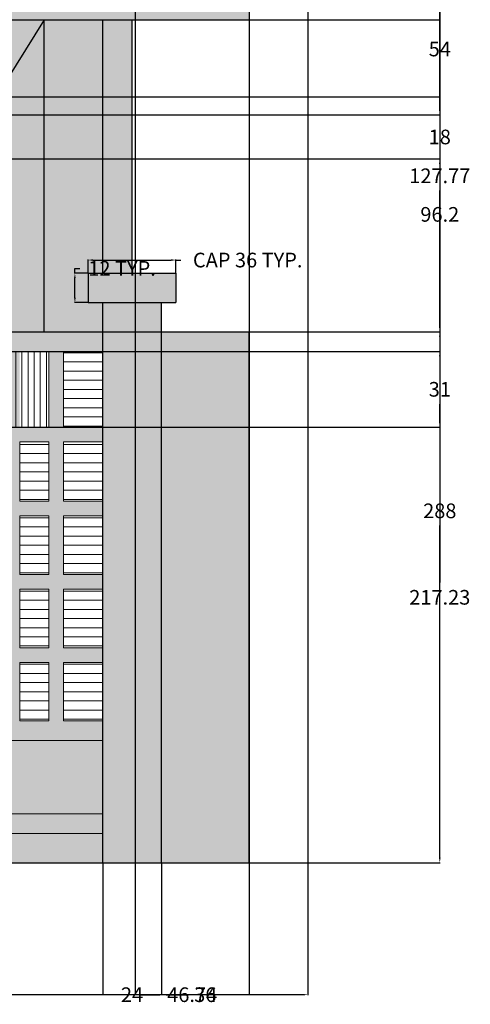
# Model space of a CAD drawing. Units: inches. Extents: x 180 to 1069, y 71 to 1267.
# Tile 5 of 8: x 884 to 1069, y 71 to 474. Entities that reach past the tile are written whole.
import ezdxf

# ---------------------------------------------------------------- set-up
doc = ezdxf.new("R2010")
doc.units = ezdxf.units.IN
doc.header["$MEASUREMENT"] = 0
for name, color, linetype, lineweight in [('A-ANNO-DIMS', 2, 'Continuous', 18), ('A-COLS', 7, 'Continuous', 25), ('A-DOOR-GATE', 7, 'Continuous', 18), ('A-DOOR-PANL-PATT', 25, 'Continuous', 13), ('A-WALL', 7, 'Continuous', 30)]:
    doc.layers.add(name, color=color, linetype=linetype, lineweight=lineweight)
for name, color, linetype, lineweight, true_color in [('A-DOOR-GATE-PATT', 18, 'Continuous', 13, 0x000000), ('A-DOOR-HARD-PATT', 8, 'Continuous', 13, 0x7f7f6c), ('A-ELEV-FRAM-PATT', 53, 'Continuous', 13, 0xefd648), ('A-ELEV-REVL-PATT', 9, 'Continuous', 13, 0xc7c8ca), ('A-ELEV-TRIM-PATT', 7, 'Continuous', 13, 0xffffff), ('A-WALL-PATT', 253, 'Continuous', 13, 0x9f9f8e), ('A-WALL-RCSD-PATT', 251, 'Continuous', 13, 0x696959)]:
    doc.layers.add(name, color=color, linetype=linetype, lineweight=lineweight, true_color=true_color)
doc.styles.get("Standard").update_dxf_attribs({"font": 'arial.ttf'})
doc.dimstyles.get("Standard").update_dxf_attribs({"dimtxt": 6, "dimasz": 2, "dimexe": 0.18, "dimexo": 0.0625, "dimgap": 3, "dimtad": 0, "dimtih": 1, "dimtoh": 1, "dimdec": 0, "dimzin": 0, "dimdsep": 46, "dimlunit": 3, "dimtxsty": 'Standard', "dimcen": 0.09, "dimadec": 0, "dimazin": 0, "dimtfac": 1, "dimtdec": 0, "dimtofl": 0, "dimtmove": 0, "dimatfit": 3, "dimfxl": 1, "dimtolj": 1, "dimtzin": 0, "dimarcsym": 0})

# ---------------------------------------------------------------- blocks, each defined once
blk = doc.blocks.new('GATE-PIER-CAP')
for p, q in [((0, 12), (36, 12)), ((0, 12), (0, 0)), ((36, 12), (36, 0)), ((0, 0), (36, 0))]:
    blk.add_line(p, q)
blk = doc.blocks.new('GATE-LEAF-LOWER-INFILL')
for p, q in [((0, 152.23), (16, 152.23)), ((16, 152.23), (16, 128)), ((22, 152.23), (34, 152.23)), ((22, 152.23), (22, 128)), ((34, 152.23), (34, 128)), ((40, 152.23), (88, 152.23)), ((40, 152.23), (40, 128)), ((88, 152.23), (88, 128)), ((94, 152.23), (106, 152.23)), ((94, 152.23), (94, 128)), ((106, 152.23), (106, 128)), ((112, 152.23), (136, 152.23)), ((112, 152.23), (112, 128)), ((136, 152.23), (136, 128)), ((0, 128), (16, 128)), ((22, 128), (34, 128)), ((40, 128), (88, 128)), ((94, 128), (106, 128)), ((112, 128), (136, 128)), ((0, 122), (16, 122)), ((16, 122), (16, 98)), ((22, 122), (34, 122)), ((22, 122), (22, 98)), ((34, 122), (34, 98)), ((40, 122), (88, 122)), ((40, 122), (40, 98)), ((88, 122), (88, 98)), ((94, 122), (106, 122)), ((94, 122), (94, 98)), ((106, 122), (106, 98)), ((112, 122), (136, 122)), ((112, 122), (112, 98)), ((136, 122), (136, 98)), ((0, 98), (16, 98)), ((22, 98), (34, 98)), ((40, 98), (88, 98)), ((94, 98), (106, 98)), ((112, 98), (136, 98)), ((0, 92), (16, 92)), ((16, 92), (16, 68)), ((22, 92), (34, 92)), ((22, 92), (22, 68)), ((34, 92), (34, 68)), ((40, 92), (88, 92)), ((40, 92), (40, 68)), ((88, 92), (88, 68)), ((94, 92), (106, 92)), ((94, 92), (94, 68)), ((106, 92), (106, 68)), ((112, 92), (136, 92)), ((112, 92), (112, 68)), ((136, 92), (136, 68)), ((0, 68), (16, 68)), ((22, 68), (34, 68)), ((40, 68), (88, 68)), ((94, 68), (106, 68)), ((112, 68), (136, 68)), ((0, 62), (16, 62)), ((16, 62), (16, 38)), ((22, 62), (34, 62)), ((22, 62), (22, 38)), ((34, 62), (34, 38)), ((40, 62), (88, 62)), ((40, 62), (40, 38)), ((88, 62), (88, 38)), ((94, 62), (106, 62)), ((94, 62), (94, 38)), ((106, 62), (106, 38)), ((112, 62), (136, 62)), ((112, 62), (112, 38)), ((136, 62), (136, 38)), ((0, 38), (16, 38)), ((22, 38), (34, 38)), ((40, 38), (88, 38)), ((94, 38), (106, 38)), ((112, 38), (136, 38)), ((0, 30), (136, 30)), ((136, 30), (136, 0)), ((0, 0), (136, 0))]:
    blk.add_line(p, q)
blk = doc.blocks.new('*D12')
at = {"layer": 'A-ANNO-DIMS', "color": 0, "lineweight": -2, "transparency": 16777216}
for p, q in [((912.09, 370.11), (912.09, 375.63)), ((914.09, 375.45), (946.09, 375.45)), ((948.09, 370.11), (948.09, 375.63)), ((948.09, 375.45), (950.09, 375.45))]:
    blk.add_line(p, q, dxfattribs=at)
at = {"layer": 'A-ANNO-DIMS', "color": 0, "transparency": 16777216}
for points in [[(914.09, 375.78), (914.09, 375.11), (912.09, 375.45)], [(946.09, 375.78), (946.09, 375.11), (948.09, 375.45)]]:
    blk.add_solid(points, dxfattribs=at)
at = {"layer": 'Defpoints', "color": 0, "transparency": 16777216}
for p in [(948.09, 375.45), (912.09, 370.05), (948.09, 370.05)]:
    blk.add_point(p, dxfattribs=at)
at = {"layer": 'A-ANNO-DIMS', "color": 0, "transparency": 16777216, "insert": (977.44, 375.45), "char_height": 6, "attachment_point": 5}
blk.add_mtext('\\A1;CAP 36 TYP.', dxfattribs=at)
blk = doc.blocks.new('*D13')
at = {"layer": 'A-ANNO-DIMS', "color": 0, "lineweight": -2, "transparency": 16777216}
for p, q in [((906.69, 370.05), (906.69, 372.05)), ((906.69, 372.05), (908.69, 372.05)), ((912.02, 370.05), (906.51, 370.05)), ((906.69, 360.05), (906.69, 368.05)), ((912.02, 358.05), (906.51, 358.05))]:
    blk.add_line(p, q, dxfattribs=at)
at = {"layer": 'A-ANNO-DIMS', "color": 0, "transparency": 16777216}
for points in [[(906.35, 368.05), (907.02, 368.05), (906.69, 370.05)], [(906.35, 360.05), (907.02, 360.05), (906.69, 358.05)]]:
    blk.add_solid(points, dxfattribs=at)
at = {"layer": 'Defpoints', "color": 0, "transparency": 16777216}
for p in [(906.69, 370.05), (912.09, 370.05), (912.09, 358.05)]:
    blk.add_point(p, dxfattribs=at)
at = {"layer": 'A-ANNO-DIMS', "color": 0, "transparency": 16777216, "insert": (926.01, 372.05), "char_height": 6, "attachment_point": 5}
blk.add_mtext('\\A1;12 TYP.', dxfattribs=at)
blk = doc.blocks.new('*D31')
at = {"layer": 'A-ANNO-DIMS', "color": 0, "lineweight": -2, "transparency": 16777216}
for p, q in [((546.15, 416.82), (1056.28, 416.82)), ((1056.1, 414.82), (1056.1, 278.88)), ((1056.1, 130.82), (1056.1, 266.75)), ((546.15, 128.82), (1056.28, 128.82))]:
    blk.add_line(p, q, dxfattribs=at)
at = {"layer": 'A-ANNO-DIMS', "color": 0, "transparency": 16777216}
for points in [[(1055.77, 414.82), (1056.43, 414.82), (1056.1, 416.82)], [(1055.77, 130.82), (1056.43, 130.82), (1056.1, 128.82)]]:
    blk.add_solid(points, dxfattribs=at)
at = {"layer": 'Defpoints', "color": 0, "transparency": 16777216}
for p in [(546.09, 416.82), (1056.1, 416.82), (546.09, 128.82)]:
    blk.add_point(p, dxfattribs=at)
at = {"layer": 'A-ANNO-DIMS', "color": 0, "transparency": 16777216, "insert": (1056.1, 272.82), "char_height": 6, "attachment_point": 5}
blk.add_mtext('\\A1;288', dxfattribs=at)
blk = doc.blocks.new('*D32')
at = {"layer": 'A-ANNO-DIMS', "color": 0, "lineweight": -2, "transparency": 16777216}
for p, q in [((1056.1, 436.82), (1056.1, 438.82)), ((606.15, 434.82), (1056.28, 434.82)), ((546.15, 416.82), (1056.28, 416.82)), ((1056.1, 414.82), (1056.1, 412.82))]:
    blk.add_line(p, q, dxfattribs=at)
at = {"layer": 'A-ANNO-DIMS', "color": 0, "transparency": 16777216}
for points in [[(1055.77, 436.82), (1056.43, 436.82), (1056.1, 434.82)], [(1055.77, 414.82), (1056.43, 414.82), (1056.1, 416.82)]]:
    blk.add_solid(points, dxfattribs=at)
at = {"layer": 'Defpoints', "color": 0, "transparency": 16777216}
for p in [(606.09, 434.82), (1056.1, 434.82), (546.09, 416.82)]:
    blk.add_point(p, dxfattribs=at)
at = {"layer": 'A-ANNO-DIMS', "color": 0, "transparency": 16777216, "insert": (1056.1, 425.82), "char_height": 6, "attachment_point": 5}
blk.add_mtext('\\A1;18', dxfattribs=at)
blk = doc.blocks.new('*D34')
at = {"layer": 'A-ANNO-DIMS', "color": 0, "lineweight": -2, "transparency": 16777216}
for p, q in [((630.09, 128.75), (630.09, 74.62)), ((918.09, 128.75), (918.09, 74.62)), ((632.09, 74.8), (764.4, 74.8)), ((916.09, 74.8), (783.77, 74.8))]:
    blk.add_line(p, q, dxfattribs=at)
at = {"layer": 'A-ANNO-DIMS', "color": 0, "transparency": 16777216}
for points in [[(632.09, 75.14), (632.09, 74.47), (630.09, 74.8)], [(916.09, 75.14), (916.09, 74.47), (918.09, 74.8)]]:
    blk.add_solid(points, dxfattribs=at)
at = {"layer": 'Defpoints', "color": 0, "transparency": 16777216}
for p in [(630.09, 128.82), (918.09, 128.82), (918.09, 74.8)]:
    blk.add_point(p, dxfattribs=at)
at = {"layer": 'A-ANNO-DIMS', "color": 0, "transparency": 16777216, "insert": (774.09, 74.8), "char_height": 6, "attachment_point": 5}
blk.add_mtext('\\A1;288', dxfattribs=at)
blk = doc.blocks.new('*D35')
at = {"layer": 'A-ANNO-DIMS', "color": 0, "lineweight": -2, "transparency": 16777216}
for p, q in [((918.09, 128.75), (918.09, 74.62)), ((942.09, 128.75), (942.09, 74.62)), ((916.09, 74.8), (914.09, 74.8)), ((944.09, 74.8), (946.09, 74.8))]:
    blk.add_line(p, q, dxfattribs=at)
at = {"layer": 'A-ANNO-DIMS', "color": 0, "transparency": 16777216}
for points in [[(916.09, 75.14), (916.09, 74.47), (918.09, 74.8)], [(944.09, 75.14), (944.09, 74.47), (942.09, 74.8)]]:
    blk.add_solid(points, dxfattribs=at)
at = {"layer": 'Defpoints', "color": 0, "transparency": 16777216}
for p in [(918.09, 128.82), (942.09, 128.82), (942.09, 74.8)]:
    blk.add_point(p, dxfattribs=at)
at = {"layer": 'A-ANNO-DIMS', "color": 0, "transparency": 16777216, "insert": (930.09, 74.8), "char_height": 6, "attachment_point": 5}
blk.add_mtext('\\A1;24', dxfattribs=at)
blk = doc.blocks.new('*D36')
at = {"layer": 'A-ANNO-DIMS', "color": 0, "lineweight": -2, "transparency": 16777216}
for p, q in [((942.09, 128.75), (942.09, 74.62)), ((978.09, 128.75), (978.09, 74.62)), ((944.09, 74.8), (952.79, 74.8)), ((976.09, 74.8), (967.38, 74.8))]:
    blk.add_line(p, q, dxfattribs=at)
at = {"layer": 'A-ANNO-DIMS', "color": 0, "transparency": 16777216}
for points in [[(944.09, 75.14), (944.09, 74.47), (942.09, 74.8)], [(976.09, 75.14), (976.09, 74.47), (978.09, 74.8)]]:
    blk.add_solid(points, dxfattribs=at)
at = {"layer": 'Defpoints', "color": 0, "transparency": 16777216}
for p in [(942.09, 128.82), (978.09, 128.82), (978.09, 74.8)]:
    blk.add_point(p, dxfattribs=at)
at = {"layer": 'A-ANNO-DIMS', "color": 0, "transparency": 16777216, "insert": (960.09, 74.8), "char_height": 6, "attachment_point": 5}
blk.add_mtext('\\A1;36', dxfattribs=at)
blk = doc.blocks.new('*D37')
at = {"layer": 'A-ANNO-DIMS', "color": 0, "lineweight": -2, "transparency": 16777216}
for p, q in [((978.15, 346.05), (1056.28, 346.05)), ((1056.1, 344.05), (1056.1, 243.5)), ((1056.1, 130.82), (1056.1, 231.37)), ((978.15, 128.82), (1056.28, 128.82))]:
    blk.add_line(p, q, dxfattribs=at)
at = {"layer": 'A-ANNO-DIMS', "color": 0, "transparency": 16777216}
for points in [[(1055.77, 344.05), (1056.43, 344.05), (1056.1, 346.05)], [(1055.77, 130.82), (1056.43, 130.82), (1056.1, 128.82)]]:
    blk.add_solid(points, dxfattribs=at)
at = {"layer": 'Defpoints', "color": 0, "transparency": 16777216}
for p in [(978.09, 346.05), (1056.1, 346.05), (978.09, 128.82)]:
    blk.add_point(p, dxfattribs=at)
at = {"layer": 'A-ANNO-DIMS', "color": 0, "transparency": 16777216, "insert": (1056.1, 237.43), "char_height": 6, "attachment_point": 5}
blk.add_mtext('\\A1;217.23', dxfattribs=at)
blk = doc.blocks.new('*D38')
at = {"layer": 'A-ANNO-DIMS', "color": 0, "lineweight": -2, "transparency": 16777216}
for p, q in [((978.15, 473.82), (1056.28, 473.82)), ((1056.1, 471.82), (1056.1, 415.94)), ((1056.1, 348.05), (1056.1, 403.92)), ((978.15, 346.05), (1056.28, 346.05))]:
    blk.add_line(p, q, dxfattribs=at)
at = {"layer": 'A-ANNO-DIMS', "color": 0, "transparency": 16777216}
for points in [[(1055.77, 471.82), (1056.43, 471.82), (1056.1, 473.82)], [(1055.77, 348.05), (1056.43, 348.05), (1056.1, 346.05)]]:
    blk.add_solid(points, dxfattribs=at)
at = {"layer": 'Defpoints', "color": 0, "transparency": 16777216}
for p in [(978.09, 473.82), (1056.1, 473.82), (978.09, 346.05)]:
    blk.add_point(p, dxfattribs=at)
at = {"layer": 'A-ANNO-DIMS', "color": 0, "transparency": 16777216, "insert": (1056.1, 409.93), "char_height": 6, "attachment_point": 5}
blk.add_mtext('\\A1;127.77', dxfattribs=at)
blk = doc.blocks.new('*D41')
at = {"layer": 'A-ANNO-DIMS', "color": 0, "lineweight": -2, "transparency": 16777216}
for p, q in [((736.15, 338.05), (1056.28, 338.05)), ((1056.1, 336.05), (1056.1, 328.61)), ((1056.1, 309.05), (1056.1, 316.48)), ((736.15, 307.05), (1056.28, 307.05))]:
    blk.add_line(p, q, dxfattribs=at)
at = {"layer": 'A-ANNO-DIMS', "color": 0, "transparency": 16777216}
for points in [[(1055.77, 336.05), (1056.43, 336.05), (1056.1, 338.05)], [(1055.77, 309.05), (1056.43, 309.05), (1056.1, 307.05)]]:
    blk.add_solid(points, dxfattribs=at)
at = {"layer": 'Defpoints', "color": 0, "transparency": 16777216}
for p in [(736.09, 338.05), (736.09, 307.05), (1056.1, 307.05)]:
    blk.add_point(p, dxfattribs=at)
at = {"layer": 'A-ANNO-DIMS', "color": 0, "transparency": 16777216, "insert": (1056.1, 322.55), "char_height": 6, "attachment_point": 5}
blk.add_mtext('\\A1;31', dxfattribs=at)
blk = doc.blocks.new('*D47')
at = {"layer": 'A-ANNO-DIMS', "color": 0, "lineweight": -2, "transparency": 16777216}
for p, q in [((825.96, 442.24), (1056.28, 442.24)), ((1056.1, 440.24), (1056.1, 400.21)), ((1056.1, 348.05), (1056.1, 388.08)), ((825.96, 346.05), (1056.28, 346.05))]:
    blk.add_line(p, q, dxfattribs=at)
at = {"layer": 'A-ANNO-DIMS', "color": 0, "transparency": 16777216}
for points in [[(1055.77, 440.24), (1056.43, 440.24), (1056.1, 442.24)], [(1055.77, 348.05), (1056.43, 348.05), (1056.1, 346.05)]]:
    blk.add_solid(points, dxfattribs=at)
at = {"layer": 'Defpoints', "color": 0, "transparency": 16777216}
for p in [(825.89, 442.24), (1056.1, 442.24), (825.89, 346.05)]:
    blk.add_point(p, dxfattribs=at)
at = {"layer": 'A-ANNO-DIMS', "color": 0, "transparency": 16777216, "insert": (1056.1, 394.14), "char_height": 6, "attachment_point": 5}
blk.add_mtext('\\A1;96.2', dxfattribs=at)
blk = doc.blocks.new('*D59')
at = {"layer": 'A-ANNO-DIMS', "color": 0, "lineweight": -2, "transparency": 16777216}
for p, q in [((606.15, 1010.82), (1056.28, 1010.82)), ((1056.1, 1008.82), (1056.1, 728.88)), ((1056.1, 436.82), (1056.1, 716.75)), ((606.15, 434.82), (1056.28, 434.82))]:
    blk.add_line(p, q, dxfattribs=at)
at = {"layer": 'A-ANNO-DIMS', "color": 0, "transparency": 16777216}
for points in [[(1055.77, 1008.82), (1056.43, 1008.82), (1056.1, 1010.82)], [(1055.77, 436.82), (1056.43, 436.82), (1056.1, 434.82)]]:
    blk.add_solid(points, dxfattribs=at)
at = {"layer": 'Defpoints', "color": 0, "transparency": 16777216}
for p in [(606.09, 1010.82), (1056.1, 1010.82), (606.09, 434.82)]:
    blk.add_point(p, dxfattribs=at)
at = {"layer": 'A-ANNO-DIMS', "color": 0, "transparency": 16777216, "insert": (1056.1, 722.82), "char_height": 6, "attachment_point": 5}
blk.add_mtext('\\A1;576', dxfattribs=at)
blk = doc.blocks.new('*D60')
at = {"layer": 'A-ANNO-DIMS', "color": 0, "lineweight": -2, "transparency": 16777216}
for p, q in [((498.15, 488.82), (1056.28, 488.82)), ((1056.1, 486.82), (1056.1, 467.87)), ((1056.1, 436.82), (1056.1, 455.76)), ((606.15, 434.82), (1056.28, 434.82))]:
    blk.add_line(p, q, dxfattribs=at)
at = {"layer": 'A-ANNO-DIMS', "color": 0, "transparency": 16777216}
for points in [[(1055.77, 486.82), (1056.43, 486.82), (1056.1, 488.82)], [(1055.77, 436.82), (1056.43, 436.82), (1056.1, 434.82)]]:
    blk.add_solid(points, dxfattribs=at)
at = {"layer": 'Defpoints', "color": 0, "transparency": 16777216}
for p in [(498.09, 488.82), (606.09, 434.82), (1056.1, 434.82)]:
    blk.add_point(p, dxfattribs=at)
at = {"layer": 'A-ANNO-DIMS', "color": 0, "transparency": 16777216, "insert": (1056.1, 461.82), "char_height": 6, "attachment_point": 5}
blk.add_mtext('\\A1;54', dxfattribs=at)
blk = doc.blocks.new('*D68')
at = {"layer": 'A-ANNO-DIMS', "color": 0, "lineweight": -2, "transparency": 16777216}
for p, q in [((702.09, 557.75), (702.09, 74.62)), ((1002.09, 557.75), (1002.09, 74.62)), ((704.09, 74.8), (842.47, 74.8)), ((1000.09, 74.8), (861.7, 74.8))]:
    blk.add_line(p, q, dxfattribs=at)
at = {"layer": 'A-ANNO-DIMS', "color": 0, "transparency": 16777216}
for points in [[(704.09, 75.14), (704.09, 74.47), (702.09, 74.8)], [(1000.09, 75.14), (1000.09, 74.47), (1002.09, 74.8)]]:
    blk.add_solid(points, dxfattribs=at)
at = {"layer": 'Defpoints', "color": 0, "transparency": 16777216}
for p in [(702.09, 557.82), (1002.09, 557.82), (1002.09, 74.8)]:
    blk.add_point(p, dxfattribs=at)
at = {"layer": 'A-ANNO-DIMS', "color": 0, "transparency": 16777216, "insert": (852.09, 74.8), "char_height": 6, "attachment_point": 5}
blk.add_mtext('\\A1;300', dxfattribs=at)
blk = doc.blocks.new('*D79')
at = {"layer": 'A-ANNO-DIMS', "color": 0, "lineweight": -2, "transparency": 16777216}
for p, q in [((931.35, 647.75), (931.35, 74.62)), ((978.09, 647.75), (978.09, 74.62)), ((933.35, 74.8), (941.49, 74.8)), ((976.09, 74.8), (967.95, 74.8))]:
    blk.add_line(p, q, dxfattribs=at)
at = {"layer": 'A-ANNO-DIMS', "color": 0, "transparency": 16777216}
for points in [[(933.35, 75.14), (933.35, 74.47), (931.35, 74.8)], [(976.09, 75.14), (976.09, 74.47), (978.09, 74.8)]]:
    blk.add_solid(points, dxfattribs=at)
at = {"layer": 'Defpoints', "color": 0, "transparency": 16777216}
for p in [(931.35, 647.82), (978.09, 647.82), (978.09, 74.8)]:
    blk.add_point(p, dxfattribs=at)
at = {"layer": 'A-ANNO-DIMS', "color": 0, "transparency": 16777216, "insert": (954.72, 74.8), "char_height": 6, "attachment_point": 5}
blk.add_mtext('\\A1;46.74', dxfattribs=at)

msp = doc.modelspace()

# ---------------------------------------------------------------- hatches: boundary and pattern name
at = {"layer": 'A-DOOR-GATE-PATT'}
h = msp.add_hatch(color=256, dxfattribs=at)
h.dxf.hatch_style = 1
h.paths.add_polyline_path([(772.0875, 346.0477), (630.0875, 346.0477), (630.0875, 338.0477), (646.0875, 338.0477), (646.0875, 307.0477), (630.0875, 307.0477), (630.0875, 301.0477), (646.0875, 301.0477), (646.0875, 276.8159), (630.0875, 276.8159), (630.0875, 270.8159), (646.0875, 270.8159), (646.0875, 246.8159), (630.0875, 246.8159), (630.0875, 240.8159), (646.0875, 240.8159), (646.0875, 216.8159), (630.0875, 216.8159), (630.0875, 210.8159), (646.0875, 210.8159), (646.0875, 186.8159), (630.0875, 186.8159), (630.0875, 178.8159), (766.0875, 178.8159), (766.0875, 148.8159), (630.0875, 148.8159), (630.0875, 140.8159), (772.0875, 140.8159)])
h.paths.add_polyline_path([(670.0875, 338.0477), (718.0875, 338.0477), (718.0875, 307.0477), (670.0875, 307.0477)], flags=16)
h.paths.add_polyline_path([(664.0875, 338.0477), (664.0875, 307.0477), (652.0875, 307.0477), (652.0875, 338.0477)], flags=16)
h.paths.add_polyline_path([(670.0875, 301.0477), (718.0875, 301.0477), (718.0875, 276.8159), (670.0875, 276.8159)], flags=16)
h.paths.add_polyline_path([(664.0875, 301.0477), (664.0875, 276.8159), (652.0875, 276.8159), (652.0875, 301.0477)], flags=16)
h.paths.add_polyline_path([(724.0875, 338.0477), (736.0875, 338.0477), (736.0875, 307.0477), (724.0875, 307.0477)], flags=16)
h.paths.add_polyline_path([(724.0875, 301.0477), (736.0875, 301.0477), (736.0875, 276.8159), (724.0875, 276.8159)], flags=16)
h.paths.add_polyline_path([(670.0875, 270.8159), (718.0875, 270.8159), (718.0875, 246.8159), (670.0875, 246.8159)], flags=16)
h.paths.add_polyline_path([(664.0875, 270.8159), (664.0875, 246.8159), (652.0875, 246.8159), (652.0875, 270.8159)], flags=16)
h.paths.add_polyline_path([(742.0875, 338.0477), (766.0875, 338.0477), (766.0875, 307.0477), (742.0875, 307.0477)], flags=16)
h.paths.add_polyline_path([(742.0875, 301.0477), (766.0875, 301.0477), (766.0875, 276.8159), (742.0875, 276.8159)], flags=16)
h.paths.add_polyline_path([(724.0875, 270.8159), (736.0875, 270.8159), (736.0875, 246.8159), (724.0875, 246.8159)], flags=16)
h.paths.add_polyline_path([(670.0875, 240.8159), (718.0875, 240.8159), (718.0875, 216.8159), (670.0875, 216.8159)], flags=16)
h.paths.add_polyline_path([(664.0875, 240.8159), (664.0875, 216.8159), (652.0875, 216.8159), (652.0875, 240.8159)], flags=16)
h.paths.add_polyline_path([(742.0875, 270.8159), (766.0875, 270.8159), (766.0875, 246.8159), (742.0875, 246.8159)], flags=16)
h.paths.add_polyline_path([(724.0875, 240.8159), (736.0875, 240.8159), (736.0875, 216.8159), (724.0875, 216.8159)], flags=16)
h.paths.add_polyline_path([(742.0875, 240.8159), (766.0875, 240.8159), (766.0875, 216.8159), (742.0875, 216.8159)], flags=16)
h.paths.add_polyline_path([(670.0875, 210.8159), (718.0875, 210.8159), (718.0875, 186.8159), (670.0875, 186.8159)], flags=16)
h.paths.add_polyline_path([(664.0875, 210.8159), (664.0875, 186.8159), (652.0875, 186.8159), (652.0875, 210.8159)], flags=16)
h.paths.add_polyline_path([(724.0875, 210.8159), (736.0875, 210.8159), (736.0875, 186.8159), (724.0875, 186.8159)], flags=16)
h.paths.add_polyline_path([(742.0875, 210.8159), (766.0875, 210.8159), (766.0875, 186.8159), (742.0875, 186.8159)], flags=16)
h.paths.add_polyline_path([(918.0875, 346.0477), (776.0875, 346.0477), (776.0875, 140.8159), (918.0875, 140.8159), (918.0875, 148.8159), (782.0875, 148.8159), (782.0875, 178.8159), (918.0875, 178.8159), (918.0875, 186.8159), (902.0875, 186.8159), (902.0875, 210.8159), (918.0875, 210.8159), (918.0875, 216.8159), (902.0875, 216.8159), (902.0875, 240.8159), (918.0875, 240.8159), (918.0875, 246.8159), (902.0875, 246.8159), (902.0875, 270.8159), (918.0875, 270.8159), (918.0875, 276.8159), (902.0875, 276.8159), (902.0875, 301.0477), (918.0875, 301.0477), (918.0875, 307.0477), (902.0875, 307.0477), (902.0875, 338.0477), (918.0875, 338.0477)])
h.paths.add_polyline_path([(782.0875, 338.0477), (806.0875, 338.0477), (806.0875, 307.0477), (782.0875, 307.0477)], flags=16)
h.paths.add_polyline_path([(812.0875, 338.0477), (824.0875, 338.0477), (824.0875, 307.0477), (812.0875, 307.0477)], flags=16)
h.paths.add_polyline_path([(782.0875, 301.0477), (806.0875, 301.0477), (806.0875, 276.8159), (782.0875, 276.8159)], flags=16)
h.paths.add_polyline_path([(830.0875, 338.0477), (878.0875, 338.0477), (878.0875, 307.0477), (830.0875, 307.0477)], flags=16)
h.paths.add_polyline_path([(812.0875, 301.0477), (824.0875, 301.0477), (824.0875, 276.8159), (812.0875, 276.8159)], flags=16)
h.paths.add_polyline_path([(830.0875, 301.0477), (878.0875, 301.0477), (878.0875, 276.8159), (830.0875, 276.8159)], flags=16)
h.paths.add_polyline_path([(782.0875, 270.8159), (806.0875, 270.8159), (806.0875, 246.8159), (782.0875, 246.8159)], flags=16)
h.paths.add_polyline_path([(812.0875, 270.8159), (824.0875, 270.8159), (824.0875, 246.8159), (812.0875, 246.8159)], flags=16)
h.paths.add_polyline_path([(830.0875, 270.8159), (878.0875, 270.8159), (878.0875, 246.8159), (830.0875, 246.8159)], flags=16)
h.paths.add_polyline_path([(782.0875, 240.8159), (806.0875, 240.8159), (806.0875, 216.8159), (782.0875, 216.8159)], flags=16)
h.paths.add_polyline_path([(884.0875, 338.0477), (896.0875, 338.0477), (896.0875, 307.0477), (884.0875, 307.0477)], flags=16)
h.paths.add_polyline_path([(812.0875, 240.8159), (824.0875, 240.8159), (824.0875, 216.8159), (812.0875, 216.8159)], flags=16)
h.paths.add_polyline_path([(884.0875, 301.0477), (896.0875, 301.0477), (896.0875, 276.8159), (884.0875, 276.8159)], flags=16)
h.paths.add_polyline_path([(830.0875, 240.8159), (878.0875, 240.8159), (878.0875, 216.8159), (830.0875, 216.8159)], flags=16)
h.paths.add_polyline_path([(884.0875, 270.8159), (896.0875, 270.8159), (896.0875, 246.8159), (884.0875, 246.8159)], flags=16)
h.paths.add_polyline_path([(782.0875, 210.8159), (806.0875, 210.8159), (806.0875, 186.8159), (782.0875, 186.8159)], flags=16)
h.paths.add_polyline_path([(812.0875, 210.8159), (824.0875, 210.8159), (824.0875, 186.8159), (812.0875, 186.8159)], flags=16)
h.paths.add_polyline_path([(830.0875, 210.8159), (878.0875, 210.8159), (878.0875, 186.8159), (830.0875, 186.8159)], flags=16)
h.paths.add_polyline_path([(884.0875, 240.8159), (896.0875, 240.8159), (896.0875, 216.8159), (884.0875, 216.8159)], flags=16)
h.paths.add_polyline_path([(884.0875, 210.8159), (896.0875, 210.8159), (896.0875, 186.8159), (884.0875, 186.8159)], flags=16)
h = msp.add_hatch(dxfattribs=at)
h.set_pattern_fill('ANSI31', color=256, scale=30, angle=135)
h.paths.add_polyline_path([(646.0875, 338.0477), (630.0875, 338.0477), (630.0875, 307.0477), (646.0875, 307.0477)])
h.paths.add_polyline_path([(646.0875, 301.0477), (630.0875, 301.0477), (630.0875, 276.8159), (646.0875, 276.8159)])
h.paths.add_polyline_path([(664.0875, 301.0477), (652.0875, 301.0477), (652.0875, 276.8159), (664.0875, 276.8159)])
h.paths.add_polyline_path([(664.0875, 270.8159), (652.0875, 270.8159), (652.0875, 246.8159), (664.0875, 246.8159)])
h.paths.add_polyline_path([(646.0875, 270.8159), (630.0875, 270.8159), (630.0875, 246.8159), (646.0875, 246.8159)])
h.paths.add_polyline_path([(646.0875, 240.8159), (630.0875, 240.8159), (630.0875, 216.8159), (646.0875, 216.8159)])
h.paths.add_polyline_path([(664.0875, 240.8159), (652.0875, 240.8159), (652.0875, 216.8159), (664.0875, 216.8159)])
h.paths.add_polyline_path([(664.0875, 210.8159), (652.0875, 210.8159), (652.0875, 186.8159), (664.0875, 186.8159)])
h.paths.add_polyline_path([(646.0875, 210.8159), (630.0875, 210.8159), (630.0875, 186.8159), (646.0875, 186.8159)])
h.paths.add_polyline_path([(736.0875, 301.0477), (724.0875, 301.0477), (724.0875, 276.8159), (736.0875, 276.8159)])
h.paths.add_polyline_path([(766.0875, 301.0477), (742.0875, 301.0477), (742.0875, 276.8159), (766.0875, 276.8159)])
h.paths.add_polyline_path([(766.0875, 270.8159), (742.0875, 270.8159), (742.0875, 246.8159), (766.0875, 246.8159)])
h.paths.add_polyline_path([(766.0875, 338.0477), (742.0875, 338.0477), (742.0875, 307.0477), (766.0875, 307.0477)])
h.paths.add_polyline_path([(736.0875, 270.8159), (724.0875, 270.8159), (724.0875, 246.8159), (736.0875, 246.8159)])
h.paths.add_polyline_path([(736.0875, 240.8159), (724.0875, 240.8159), (724.0875, 216.8159), (736.0875, 216.8159)])
h.paths.add_polyline_path([(766.0875, 240.8159), (742.0875, 240.8159), (742.0875, 216.8159), (766.0875, 216.8159)])
h.paths.add_polyline_path([(766.0875, 210.8159), (742.0875, 210.8159), (742.0875, 186.8159), (766.0875, 186.8159)])
h.paths.add_polyline_path([(736.0875, 210.8159), (724.0875, 210.8159), (724.0875, 186.8159), (736.0875, 186.8159)])
h.paths.add_polyline_path([(806.0875, 210.8159), (782.0875, 210.8159), (782.0875, 186.8159), (806.0875, 186.8159)])
h.paths.add_polyline_path([(806.0875, 240.8159), (782.0875, 240.8159), (782.0875, 216.8159), (806.0875, 216.8159)])
h.paths.add_polyline_path([(806.0875, 270.8159), (782.0875, 270.8159), (782.0875, 246.8159), (806.0875, 246.8159)])
h.paths.add_polyline_path([(806.0875, 301.0477), (782.0875, 301.0477), (782.0875, 276.8159), (806.0875, 276.8159)])
h.paths.add_polyline_path([(806.0875, 338.0477), (782.0875, 338.0477), (782.0875, 307.0477), (806.0875, 307.0477)])
h.paths.add_polyline_path([(824.0875, 301.0477), (812.0875, 301.0477), (812.0875, 276.8159), (824.0875, 276.8159)])
h.paths.add_polyline_path([(824.0875, 270.8159), (812.0875, 270.8159), (812.0875, 246.8159), (824.0875, 246.8159)])
h.paths.add_polyline_path([(824.0875, 240.8159), (812.0875, 240.8159), (812.0875, 216.8159), (824.0875, 216.8159)])
h.paths.add_polyline_path([(824.0875, 210.8159), (812.0875, 210.8159), (812.0875, 186.8159), (824.0875, 186.8159)])
h.paths.add_polyline_path([(918.0875, 338.0477), (902.0875, 338.0477), (902.0875, 307.0477), (918.0875, 307.0477)])
h.paths.add_polyline_path([(918.0875, 301.0477), (902.0875, 301.0477), (902.0875, 276.8159), (918.0875, 276.8159)])
h.paths.add_polyline_path([(918.0875, 270.8159), (902.0875, 270.8159), (902.0875, 246.8159), (918.0875, 246.8159)])
h.paths.add_polyline_path([(918.0875, 240.8159), (902.0875, 240.8159), (902.0875, 216.8159), (918.0875, 216.8159)])
h.paths.add_polyline_path([(918.0875, 210.8159), (902.0875, 210.8159), (902.0875, 186.8159), (918.0875, 186.8159)])
h.paths.add_polyline_path([(896.0875, 210.8159), (884.0875, 210.8159), (884.0875, 186.8159), (896.0875, 186.8159)])
h.paths.add_polyline_path([(896.0875, 240.8159), (884.0875, 240.8159), (884.0875, 216.8159), (896.0875, 216.8159)])
h.paths.add_polyline_path([(896.0875, 270.8159), (884.0875, 270.8159), (884.0875, 246.8159), (896.0875, 246.8159)])
h.paths.add_polyline_path([(896.0875, 301.0477), (884.0875, 301.0477), (884.0875, 276.8159), (896.0875, 276.8159)])
h = msp.add_hatch(dxfattribs=at)
h.set_pattern_fill('ANSI31', color=256, scale=20, angle=45)
h.paths.add_polyline_path([(736.0875, 338.0477), (724.0875, 338.0477), (664.0875, 338.0477), (652.0875, 338.0477), (652.0875, 307.0477), (664.0875, 307.0477), (724.0875, 307.0477), (736.0875, 307.0477)])
h.paths.add_polyline_path([(896.0875, 338.0477), (884.0875, 338.0477), (824.0875, 338.0477), (812.0875, 338.0477), (812.0875, 307.0477), (830.0875, 307.0477), (884.0875, 307.0477), (896.0875, 307.0477)])
at = {"layer": 'A-DOOR-HARD-PATT'}
h = msp.add_hatch(color=256, dxfattribs=at)
h.dxf.hatch_style = 1
h.paths.add_polyline_path([(918.0875, 140.8159), (776.0875, 140.8159), (772.0875, 140.8159), (630.0875, 140.8159), (630.0875, 128.8159), (918.0875, 128.8159)])
at = {"layer": 'A-DOOR-PANL-PATT'}
h = msp.add_hatch(color=256, dxfattribs=at)
h.dxf.hatch_style = 1
h.paths.add_polyline_path([(766.0875, 178.8159), (630.0875, 178.8159), (630.0875, 148.8159), (766.0875, 148.8159)])
h.paths.add_polyline_path([(918.0875, 178.8159), (782.0875, 178.8159), (782.0875, 148.8159), (918.0875, 148.8159)])
h.paths.add_polyline_path([(878.0875, 210.8159), (830.0875, 210.8159), (830.0875, 186.8159), (878.0875, 186.8159)])
h.paths.add_polyline_path([(878.0875, 240.8159), (830.0875, 240.8159), (830.0875, 216.8159), (878.0875, 216.8159)])
h.paths.add_polyline_path([(878.0875, 270.8159), (830.0875, 270.8159), (830.0875, 246.8159), (878.0875, 246.8159)])
h.paths.add_polyline_path([(878.0875, 301.0477), (830.0875, 301.0477), (830.0875, 276.8159), (878.0875, 276.8159)])
h.paths.add_polyline_path([(718.0875, 301.0477), (670.0875, 301.0477), (670.0875, 276.8159), (718.0875, 276.8159)])
h.paths.add_polyline_path([(718.0875, 270.8159), (670.0875, 270.8159), (670.0875, 246.8159), (718.0875, 246.8159)])
h.paths.add_polyline_path([(718.0875, 240.8159), (670.0875, 240.8159), (670.0875, 216.8159), (718.0875, 216.8159)])
h.paths.add_polyline_path([(718.0875, 210.8159), (670.0875, 210.8159), (670.0875, 186.8159), (718.0875, 186.8159)])
at = {"layer": 'A-ELEV-FRAM-PATT'}
h = msp.add_hatch(color=256, dxfattribs=at)
h.dxf.hatch_style = 1
h.paths.add_polyline_path([(354.0875, 1184.8159), (654.0875, 1184.8159), (654.0875, 974.8159), (726.0875, 974.8159), (726.0875, 1208.8159), (288.0875, 1208.8159), (288.0875, 897.6348), (304.7188, 897.6348), (304.7188, 883.4805), (288.0875, 883.4805), (288.0875, 866.8025), (304.7188, 866.8025), (304.7188, 852.6482), (288.0875, 852.6482), (288.0875, 835.9702), (304.7188, 835.9702), (304.7188, 821.8159), (288.0875, 821.8159), (288.0875, 805.1379), (304.7188, 805.1379), (304.7188, 790.9836), (288.0875, 790.9836), (288.0875, 774.3056), (304.7188, 774.3056), (304.7188, 760.1513), (288.0875, 760.1513), (288.0875, 743.4733), (304.7188, 743.4733), (304.7188, 729.319), (288.0875, 729.319), (288.0875, 434.8159), (354.0875, 434.8159), (354.0875, 456.1177), (317.1892, 456.1177), (317.1892, 516.1177), (354.0875, 516.1177), (354.0875, 924.0304), (317.1892, 924.0304), (317.1892, 984.0304), (354.0875, 984.0304)])
h.paths.add_polyline_path([(1002.0875, 869.8159), (702.0875, 869.8159), (702.0875, 791.8159), (726.0875, 791.8159), (726.0875, 845.8159), (978.0875, 845.8159), (978.0875, 581.8159), (726.0875, 581.8159), (726.0875, 647.8159), (702.0875, 647.8159), (702.0875, 557.8159), (1002.0875, 557.8159)])
h.paths.add_polyline_path([(906.0875, 1080.2003), (882.0875, 1080.2003), (882.0875, 1056.2003), (906.0875, 1056.2003)])
h.paths.add_polyline_path([(906.0875, 996.2003), (882.0875, 996.2003), (882.0875, 972.2003), (906.0875, 972.2003)])
h.paths.add_polyline_path([(636.5273, 869.8159), (612.5273, 869.8159), (612.5273, 845.8159), (636.5273, 845.8159)], flags=17)
h.paths.add_polyline_path([(682.6602, 869.8159), (658.6602, 869.8159), (658.6602, 845.8159), (682.6602, 845.8159)], flags=17)
h.paths.add_polyline_path([(636.5273, 581.8159), (612.5273, 581.8159), (612.5273, 557.8159), (636.5273, 557.8159)], flags=17)
h.paths.add_polyline_path([(682.6602, 581.8159), (658.6602, 581.8159), (658.6602, 557.8159), (682.6602, 557.8159)], flags=17)
h.paths.add_polyline_path([(942.0875, 358.0477), (918.0875, 358.0477), (918.0875, 128.8159), (942.0875, 128.8159)])
h.paths.add_polyline_path([(630.0875, 358.0477), (606.0875, 358.0477), (606.0875, 128.8159), (630.0875, 128.8159)])
h = msp.add_hatch(color=256, dxfattribs=at)
h.dxf.hatch_style = 1
h.paths.add_polyline_path([(918.0875, 473.8159), (894.0875, 473.8159), (894.0875, 346.0477), (918.0875, 346.0477), (918.0875, 358.0477), (912.0875, 358.0477), (912.0875, 370.0477), (918.0875, 370.0477)])
at = {"layer": 'A-ELEV-REVL-PATT'}
h = msp.add_hatch(color=256, dxfattribs=at)
h.dxf.hatch_style = 1
h.paths.add_polyline_path([(978.0875, 791.8159), (960.2423, 791.8159), (907.3511, 731.8159), (931.3511, 731.8159), (931.3511, 647.8159), (978.0875, 647.8159)])
h.paths.add_polyline_path([(978.0875, 346.0477), (942.0875, 346.0477), (942.0875, 128.8159), (978.0875, 128.8159)])
at = {"layer": 'A-ELEV-TRIM-PATT'}
h = msp.add_hatch(color=256, dxfattribs=at)
h.dxf.hatch_style = 1
h.paths.add_polyline_path([(467.1892, 516.1177), (317.1892, 516.1177), (317.1892, 456.1177), (467.1892, 456.1177)])
h.paths.add_polyline_path([(458.1892, 507.1177), (458.1892, 465.1177), (326.1892, 465.1177), (326.1892, 507.1177)], flags=16)
h.paths.add_polyline_path([(354.0875, 816.0741), (354.0875, 804.0741), (426.0875, 804.0741), (426.0875, 636.0741), (354.0875, 636.0741), (354.0875, 624.0741), (438.0875, 624.0741), (438.0875, 816.0741)])
h.paths.add_polyline_path([(317.1892, 924.0304), (467.1892, 924.0304), (467.1892, 984.0304), (317.1892, 984.0304)])
h.paths.add_polyline_path([(326.1892, 933.0304), (326.1892, 975.0304), (458.1892, 975.0304), (458.1892, 933.0304)], flags=16)
h.paths.add_polyline_path([(304.7188, 897.6348), (262.2193, 897.6348), (262.2193, 883.4805), (304.7188, 883.4805)])
h.paths.add_polyline_path([(304.7188, 866.8025), (262.2193, 866.8025), (262.2193, 852.6482), (304.7188, 852.6482)])
h.paths.add_polyline_path([(304.7188, 835.9702), (262.2193, 835.9702), (262.2193, 821.8159), (304.7188, 821.8159)])
h.paths.add_polyline_path([(304.7188, 805.1379), (262.2193, 805.1379), (262.2193, 790.9836), (304.7188, 790.9836)])
h.paths.add_polyline_path([(304.7188, 774.3056), (262.2193, 774.3056), (262.2193, 760.1513), (304.7188, 760.1513)])
h.paths.add_polyline_path([(304.7188, 743.4733), (262.2193, 743.4733), (262.2193, 729.319), (304.7188, 729.319)])
h.paths.add_polyline_path([(600.0875, 370.0477), (600.0875, 358.0477), (636.0875, 358.0477), (636.0875, 370.0477)])
h.paths.add_polyline_path([(912.0875, 370.0477), (912.0875, 358.0477), (948.0875, 358.0477), (948.0875, 370.0477)])
at = {"layer": 'A-WALL-PATT'}
h = msp.add_hatch(color=256, dxfattribs=at)
h.dxf.hatch_style = 1
h.paths.add_polyline_path([(978.0875, 947.2513), (834.0875, 947.2513), (834.0875, 869.8159), (978.0875, 869.8159)])
h.paths.add_polyline_path([(978.0875, 557.8159), (834.0875, 557.8159), (834.0875, 473.8159), (978.0875, 473.8159)])
h.paths.add_polyline_path([(960.2423, 791.8159), (606.0875, 791.8159), (606.0875, 647.8159), (883.3511, 647.8159), (883.3511, 731.8159), (907.3511, 731.8159)])
h = msp.add_hatch(color=256, dxfattribs=at)
h.dxf.hatch_style = 1
h.paths.add_polyline_path([(894.0875, 473.8159), (825.8928, 364.2866), (825.8928, 346.0477), (894.0875, 346.0477)])
h = msp.add_hatch(color=256, dxfattribs=at)
h.dxf.hatch_style = 1
h.paths.add_polyline_path([(930.0875, 473.8159), (918.0875, 473.8159), (918.0875, 370.0477), (930.0875, 370.0477)])
at = {"layer": 'A-WALL-RCSD-PATT'}
h = msp.add_hatch(color=256, dxfattribs=at)
h.dxf.hatch_style = 1
h.paths.add_polyline_path([(741.8928, 442.2382), (825.8928, 442.2382), (825.8928, 364.2866), (894.0875, 473.8159), (606.0875, 473.8159), (606.0875, 442.2382), (690.001, 442.2382), (690.001, 346.0477), (741.8928, 346.0477)])

# ---------------------------------------------------------------- linework, layer by layer
at = {"layer": 'A-COLS'}
for p, q in [((894.0875, 346.0477), (894.0875, 473.8159)), ((918.0875, 370.0477), (918.0875, 473.8159)), ((930.0875, 370.0477), (930.0875, 473.8159)), ((918.0875, 128.8159), (918.0875, 358.0477)), ((942.0875, 128.8159), (942.0875, 358.0477))]:
    msp.add_line(p, q, dxfattribs=at)
at = {"layer": 'A-DOOR-GATE'}
for p, q in [((776.0875, 346.0477), (918.0875, 346.0477)), ((884.0875, 338.0477), (896.0875, 338.0477)), ((896.0875, 338.0477), (896.0875, 307.0477)), ((902.0875, 338.0477), (902.0875, 307.0477)), ((902.0875, 338.0477), (918.0875, 338.0477)), ((884.0875, 307.0477), (896.0875, 307.0477)), ((902.0875, 307.0477), (918.0875, 307.0477)), ((776.0875, 140.8159), (918.0875, 140.8159))]:
    msp.add_line(p, q, dxfattribs=at)
at = {"layer": 'A-WALL'}
for p, q in [((606.0875, 473.8159), (978.0875, 473.8159)), ((894.0875, 473.8159), (825.8928, 364.2866)), ((942.0875, 346.0477), (978.0875, 346.0477)), ((978.0875, 128.8159), (978.0875, 346.0477)), ((246.0875, 128.8159), (978.0875, 128.8159))]:
    msp.add_line(p, q, dxfattribs=at)

# ---------------------------------------------------------------- block references
at = {"layer": 'A-COLS'}
msp.add_blockref('GATE-PIER-CAP', (912.0875, 358.0477), dxfattribs=at)
at = {"layer": 'A-DOOR-GATE', "extrusion": (0, 0, -1), "zscale": -1}
msp.add_blockref('GATE-LEAF-LOWER-INFILL', (-918.0875, 148.8159), dxfattribs=at)

# ---------------------------------------------------------------- dimensions: what is measured, and where the dimension line sits
at = {"layer": 'A-ANNO-DIMS'}
for base, p1, p2, override, picture, middle in [((1056.101, 1010.8159), (606.0875, 434.8159), (606.0875, 1010.8159), {"dimdec": 0, "dimlfac": 1, "dimrnd": 0, "dimzin": 0, "dimdsep": 46, "dimlunit": 2}, '*D59', (1056.101, 722.8159)), ((1056.101, 434.8159), (498.0875, 488.8159), (606.0875, 434.8159), {"dimdec": 0, "dimlfac": 1, "dimrnd": 0, "dimzin": 0, "dimdsep": 46, "dimlunit": 2}, '*D60', (1056.101, 461.8159)), ((1056.101, 473.8159), (978.0875, 346.0477), (978.0875, 473.8159), {"dimdec": 2, "dimlfac": 1, "dimrnd": 0, "dimzin": 0, "dimdsep": 46, "dimlunit": 2}, '*D38', (1056.101, 409.9318)), ((1056.101, 442.2382), (825.8928, 346.0477), (825.8928, 442.2382), {"dimdec": 1, "dimlfac": 1, "dimrnd": 0, "dimzin": 0, "dimdsep": 46, "dimlunit": 2}, '*D47', (1056.101, 394.1429)), ((1056.101, 434.8159), (546.0875, 416.8159), (606.0875, 434.8159), {"dimdec": 0, "dimlfac": 1, "dimrnd": 0, "dimzin": 0, "dimdsep": 46, "dimlunit": 2}, '*D32', (1056.101, 425.8159)), ((1056.101, 416.8159), (546.0875, 128.8159), (546.0875, 416.8159), {"dimdec": 0, "dimlfac": 1, "dimrnd": 0, "dimzin": 0, "dimdsep": 46, "dimlunit": 2}, '*D31', (1056.101, 272.8159)), ((1056.101, 346.0477), (978.0875, 128.8159), (978.0875, 346.0477), {"dimdec": 2, "dimlfac": 1, "dimrnd": 0, "dimzin": 0, "dimdsep": 46, "dimlunit": 2}, '*D37', (1056.101, 237.4318)), ((1056.101, 307.0477), (736.0875, 338.0477), (736.0875, 307.0477), {"dimdec": 0, "dimlfac": 1, "dimrnd": 0, "dimzin": 0, "dimdsep": 46, "dimlunit": 2}, '*D41', (1056.101, 322.5477))]:
    dim = msp.add_linear_dim(base=base, p1=p1, p2=p2, angle=90, dimstyle='Standard', override=override, dxfattribs=at)
    dim.commit()
    dim.dimension.update_dxf_attribs({"geometry": picture, "text_midpoint": middle})
for base, p1, p2, override, picture, middle in [((978.0875, 74.8024), (931.3511, 647.8159), (978.0875, 647.8159), {"dimdec": 2, "dimlfac": 1, "dimrnd": 0, "dimzin": 0, "dimdsep": 46, "dimlunit": 2}, '*D79', (954.7193, 74.8024)), ((1002.0875, 74.8024), (702.0875, 557.8159), (1002.0875, 557.8159), {"dimdec": 0, "dimlfac": 1, "dimrnd": 0, "dimzin": 0, "dimdsep": 46, "dimlunit": 2}, '*D68', (852.0875, 74.8024)), ((918.0875, 74.8024), (630.0875, 128.8159), (918.0875, 128.8159), {"dimdec": 0, "dimlfac": 1, "dimrnd": 0, "dimzin": 0, "dimdsep": 46, "dimlunit": 2}, '*D34', (774.0875, 74.8024)), ((942.0875, 74.8024), (918.0875, 128.8159), (942.0875, 128.8159), {"dimdec": 0, "dimlfac": 1, "dimrnd": 0, "dimzin": 0, "dimdsep": 46, "dimlunit": 2}, '*D35', (930.0875, 74.8024)), ((978.0875, 74.8024), (942.0875, 128.8159), (978.0875, 128.8159), {"dimdec": 0, "dimlfac": 1, "dimrnd": 0, "dimzin": 0, "dimdsep": 46, "dimlunit": 2}, '*D36', (960.0875, 74.8024))]:
    dim = msp.add_linear_dim(base=base, p1=p1, p2=p2, dimstyle='Standard', override=override, dxfattribs=at)
    dim.commit()
    dim.dimension.update_dxf_attribs({"geometry": picture, "text_midpoint": middle})
dim = msp.add_linear_dim(base=(948.0875, 375.4477), p1=(912.0875, 370.0477), p2=(948.0875, 370.0477), text='CAP <> TYP.', dimstyle='Standard', override={"dimdec": 0, "dimlfac": 1, "dimrnd": 0, "dimzin": 0, "dimdsep": 46, "dimlunit": 2}, dxfattribs=at)
dim.commit()
dim.dimension.update_dxf_attribs({"geometry": '*D12', "text_midpoint": (977.4374, 375.4477)})
dim = msp.add_linear_dim(base=(906.6875, 370.0477), p1=(912.0875, 358.0477), p2=(912.0875, 370.0477), angle=90, text='<> TYP.', dimstyle='Standard', override={"dimdec": 0, "dimlfac": 1, "dimrnd": 0, "dimzin": 0, "dimdsep": 46, "dimlunit": 2}, dxfattribs=at)
dim.commit()
dim.dimension.update_dxf_attribs({"geometry": '*D13', "text_midpoint": (926.0081, 372.0477)})

doc.saveas('drawing.dxf')
